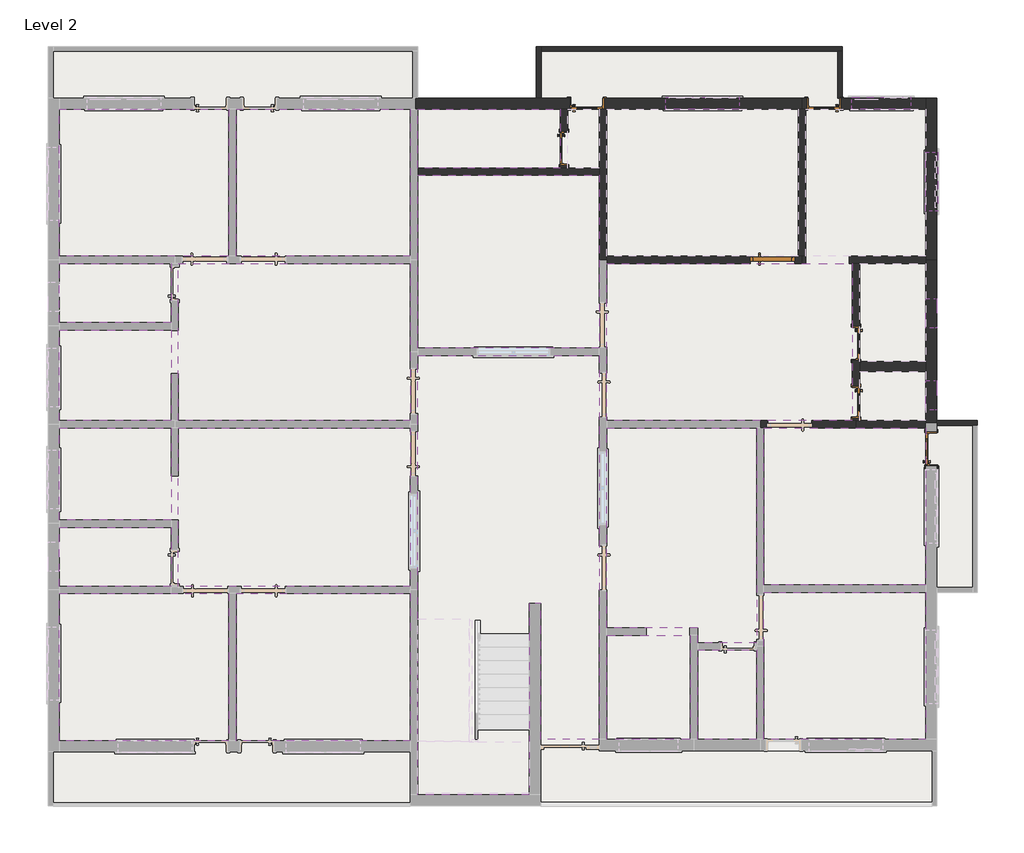
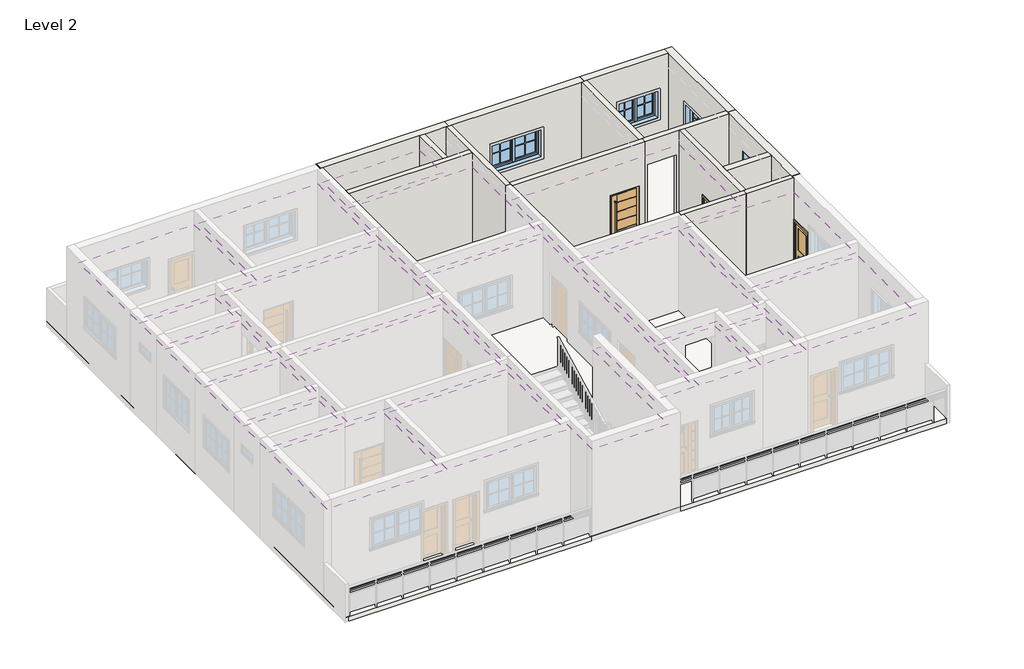
# One storey, part 3 of 5: 19 coverings, 19 walls, 7 doors, 5 windows, 1 slab.
"""IFC4 building model written with IfcOpenShell, lengths in millimetres."""

from ifc_helpers import new_model, si_unit, frame, origin, place, context, project, spatial, polyline, outline, extrude, faceted_brep, transform, mapped, element, save
from components import door_3_ad1505b7, m_door_interior_single_2_panel_wood_2_8c5b34de, door_57d9c04c, door_c5a180fb, door_5f4ff63b, door_e2914254, fixed_2_d9cafb20, m_window_awning_double_horizontal_4_0c6a2509, m_window_awning_double_horizontal_5_7c720334

model = new_model("IFC4")

# Units and contexts
model_context = context("Model", 3, world=origin())
ifc_project = project(units=[si_unit("LENGTHUNIT", "METRE", prefix="MILLI")], contexts=[model_context])

# Site, building, storey
site = spatial("IfcSite", under=ifc_project)
building = spatial("IfcBuilding", under=site)
storey = spatial("IfcBuildingStorey", under=building, Name="Level 2", Elevation=3200.4)

# Coverings
placement = place(None, origin())
element("IfcCovering", 1, ObjectType="2' x 4' ACT System", at=placement, inside=storey, context=model_context, shape_type="SweptSolid", body=[
    extrude(outline(polyline([(-22388.4847893, 20054.3922903), (-24776.0847893, 20054.3922903), (-24776.0847893, 23102.3922903), (-21270.8847893, 23102.3922903), (-21270.8847893, 20054.3922903), (-22388.4847893, 20054.3922903)])), frame((0.0, 0.0, 5943.6), z_axis=(0.0, 0.0, 1.0), x_axis=(1.0, 0.0, 0.0)), (0.0, 0.0, 1.0), 57.15),
])
element("IfcCovering", 2, ObjectType="2' x 4' ACT System", at=placement, inside=storey, context=model_context, shape_type="SweptSolid", body=[
    extrude(outline(polyline([(-21118.4847893, 23102.3922903), (-17511.6847893, 23102.3922903), (-17511.6847893, 20054.3922903), (-21118.4847893, 20054.3922903), (-21118.4847893, 23102.3922903)])), frame((0.0, 0.0, 5943.6), z_axis=(0.0, 0.0, 1.0), x_axis=(1.0, 0.0, 0.0)), (0.0, 0.0, 1.0), 57.15),
])
element("IfcCovering", 3, ObjectType="2' x 4' ACT System", at=placement, inside=storey, context=model_context, shape_type="SweptSolid", body=[
    extrude(outline(polyline([(-14412.8847893, 21883.1922903), (-17359.2847893, 21883.1922903), (-17359.2847893, 23102.3922903), (-14412.8847893, 23102.3922903), (-14412.8847893, 21883.1922903)])), frame((0.0, 0.0, 5943.6), z_axis=(0.0, 0.0, 1.0), x_axis=(1.0, 0.0, 0.0)), (0.0, 0.0, 1.0), 57.15),
])
element("IfcCovering", 4, ObjectType="2' x 4' ACT System", at=placement, inside=storey, context=model_context, shape_type="SweptSolid", body=[
    extrude(outline(polyline([(-17359.2847893, 18149.3922903), (-17359.2847893, 19978.1922903), (-17359.2847893, 21730.7922903), (-13600.0847893, 21730.7922903), (-13600.0847893, 19978.1922903), (-13600.0847893, 18149.3922903), (-17359.2847893, 18149.3922903)])), frame((0.0, 0.0, 5943.6), z_axis=(0.0, 0.0, 1.0), x_axis=(1.0, 0.0, 0.0)), (0.0, 0.0, 1.0), 57.15),
])
element("IfcCovering", 5, ObjectType="2' x 4' ACT System", at=placement, inside=storey, context=model_context, shape_type="SweptSolid", body=[
    extrude(outline(polyline([(-13447.6847893, 16650.7922903), (-13447.6847893, 19901.9922903), (-9409.0847893, 19901.9922903), (-8367.6847893, 19901.9922903), (-8367.6847893, 16650.7922903), (-10272.6847893, 16650.7922903), (-13447.6847893, 16650.7922903)])), frame((0.0, 0.0, 5943.6), z_axis=(0.0, 0.0, 1.0), x_axis=(1.0, 0.0, 0.0)), (0.0, 0.0, 1.0), 57.15),
])
element("IfcCovering", 6, ObjectType="2' x 4' ACT System", at=placement, inside=storey, context=model_context, shape_type="SweptSolid", body=[
    extrude(outline(polyline([(-6843.6847893, 16498.3922903), (-6843.6847893, 13247.1922903), (-10196.4847893, 13247.1922903), (-10196.4847893, 16498.3922903), (-8291.4847893, 16498.3922903), (-6843.6847893, 16498.3922903)])), frame((0.0, 0.0, 5943.6), z_axis=(0.0, 0.0, 1.0), x_axis=(1.0, 0.0, 0.0)), (0.0, 0.0, 1.0), 57.15),
])
element("IfcCovering", 7, ObjectType="2' x 4' ACT System", at=placement, inside=storey, context=model_context, shape_type="SweptSolid", body=[
    extrude(outline(polyline([(-6843.6847893, 13094.7922903), (-6843.6847893, 10046.7922903), (-10196.4847893, 10046.7922903), (-10196.4847893, 11977.1922903), (-10196.4847893, 13094.7922903), (-6843.6847893, 13094.7922903)])), frame((0.0, 0.0, 5943.6), z_axis=(0.0, 0.0, 1.0), x_axis=(1.0, 0.0, 0.0)), (0.0, 0.0, 1.0), 57.15),
])
element("IfcCovering", 8, ObjectType="2' x 4' ACT System", at=placement, inside=storey, context=model_context, shape_type="SweptSolid", body=[
    extrude(outline(polyline([(-11568.0847893, 10046.7922903), (-11568.0847893, 11900.9922903), (-10348.8847893, 11900.9922903), (-10348.8847893, 10046.7922903), (-11568.0847893, 10046.7922903)])), frame((0.0, 0.0, 5943.6), z_axis=(0.0, 0.0, 1.0), x_axis=(1.0, 0.0, 0.0)), (0.0, 0.0, 1.0), 57.15),
])
element("IfcCovering", 9, ObjectType="2' x 4' ACT System", at=placement, inside=storey, context=model_context, shape_type="SweptSolid", body=[
    extrude(outline(polyline([(-13447.6847893, 10046.7922903), (-13447.6847893, 12205.7922903), (-11720.4847893, 12205.7922903), (-11720.4847893, 10046.7922903), (-13447.6847893, 10046.7922903)])), frame((0.0, 0.0, 5943.6), z_axis=(0.0, 0.0, 1.0), x_axis=(1.0, 0.0, 0.0)), (0.0, 0.0, 1.0), 57.15),
])
element("IfcCovering", 10, ObjectType="2' x 4' ACT System", at=placement, inside=storey, context=model_context, shape_type="SweptSolid", body=[
    extrude(outline(polyline([(-13447.6847893, 12358.1922903), (-13447.6847893, 16498.3922903), (-10348.8847893, 16498.3922903), (-10348.8847893, 12053.3922903), (-11568.0847893, 12053.3922903), (-11568.0847893, 12358.1922903), (-13447.6847893, 12358.1922903)])), frame((0.0, 0.0, 5943.6), z_axis=(0.0, 0.0, 1.0), x_axis=(1.0, 0.0, 0.0)), (0.0, 0.0, 1.0), 57.15),
])
element("IfcCovering", 11, ObjectType="2' x 4' ACT System", at=placement, inside=storey, context=model_context, shape_type="SweptSolid", body=[
    extrude(outline(polyline([(-15047.8847893, 12866.1922903), (-15047.8847893, 8903.7922903), (-17359.2847893, 8903.7922903), (-17359.2847893, 13145.5922903), (-17359.2847893, 16574.5922903), (-17359.2847893, 17996.9922903), (-13600.0847893, 17996.9922903), (-13600.0847893, 10046.7922903), (-14819.2847893, 10046.7922903), (-14819.2847893, 12866.1922903), (-15047.8847893, 12866.1922903)])), frame((0.0, 0.0, 5943.6), z_axis=(0.0, 0.0, 1.0), x_axis=(1.0, 0.0, 0.0)), (0.0, 0.0, 1.0), 57.15),
])
element("IfcCovering", 12, ObjectType="2' x 4' ACT System", at=placement, inside=storey, context=model_context, shape_type="SweptSolid", body=[
    extrude(outline(polyline([(-17511.6847893, 13221.7922903), (-22312.2847893, 13221.7922903), (-22312.2847893, 16498.3922903), (-17511.6847893, 16498.3922903), (-17511.6847893, 13221.7922903)])), frame((0.0, 0.0, 5943.6), z_axis=(0.0, 0.0, 1.0), x_axis=(1.0, 0.0, 0.0)), (0.0, 0.0, 1.0), 57.15),
])
element("IfcCovering", 13, ObjectType="2' x 4' ACT System", at=placement, inside=storey, context=model_context, shape_type="SweptSolid", body=[
    extrude(outline(polyline([(-17511.6847893, 10021.3922903), (-21118.4847893, 10021.3922903), (-21118.4847893, 13069.3922903), (-17511.6847893, 13069.3922903), (-17511.6847893, 10021.3922903)])), frame((0.0, 0.0, 5943.6), z_axis=(0.0, 0.0, 1.0), x_axis=(1.0, 0.0, 0.0)), (0.0, 0.0, 1.0), 57.15),
])
element("IfcCovering", 14, ObjectType="2' x 4' ACT System", at=placement, inside=storey, context=model_context, shape_type="SweptSolid", body=[
    extrude(outline(polyline([(-21270.8847893, 13069.3922903), (-21270.8847893, 10021.3922903), (-24776.0847893, 10021.3922903), (-24776.0847893, 13069.3922903), (-22477.3847893, 13069.3922903), (-21270.8847893, 13069.3922903)])), frame((0.0, 0.0, 5943.6), z_axis=(0.0, 0.0, 1.0), x_axis=(1.0, 0.0, 0.0)), (0.0, 0.0, 1.0), 57.15),
])
element("IfcCovering", 15, ObjectType="2' x 4' ACT System", at=placement, inside=storey, context=model_context, shape_type="SweptSolid", body=[
    extrude(outline(polyline([(-22464.6847893, 13221.7922903), (-24776.0847893, 13221.7922903), (-24776.0847893, 14440.9922903), (-22464.6847893, 14440.9922903), (-22464.6847893, 13221.7922903)])), frame((0.0, 0.0, 5943.6), z_axis=(0.0, 0.0, 1.0), x_axis=(1.0, 0.0, 0.0)), (0.0, 0.0, 1.0), 57.15),
])
element("IfcCovering", 16, ObjectType="2' x 4' ACT System", at=placement, inside=storey, context=model_context, shape_type="SweptSolid", body=[
    extrude(outline(polyline([(-24776.0847893, 14593.3922903), (-24776.0847893, 16498.3922903), (-22464.6847893, 16498.3922903), (-22464.6847893, 14593.3922903), (-24776.0847893, 14593.3922903)])), frame((0.0, 0.0, 5943.6), z_axis=(0.0, 0.0, 1.0), x_axis=(1.0, 0.0, 0.0)), (0.0, 0.0, 1.0), 57.15),
])
element("IfcCovering", 17, ObjectType="2' x 4' ACT System", at=placement, inside=storey, context=model_context, shape_type="SweptSolid", body=[
    extrude(outline(polyline([(-22464.6847893, 18530.3922903), (-22464.6847893, 16650.7922903), (-24776.0847893, 16650.7922903), (-24776.0847893, 18530.3922903), (-22464.6847893, 18530.3922903)])), frame((0.0, 0.0, 5943.6), z_axis=(0.0, 0.0, 1.0), x_axis=(1.0, 0.0, 0.0)), (0.0, 0.0, 1.0), 57.15),
])
element("IfcCovering", 18, ObjectType="2' x 4' ACT System", at=placement, inside=storey, context=model_context, shape_type="SweptSolid", body=[
    extrude(outline(polyline([(-17511.6847893, 16650.7922903), (-22312.2847893, 16650.7922903), (-22312.2847893, 19901.9922903), (-17511.6847893, 19901.9922903), (-17511.6847893, 18073.1922903), (-17511.6847893, 16650.7922903)])), frame((0.0, 0.0, 5943.6), z_axis=(0.0, 0.0, 1.0), x_axis=(1.0, 0.0, 0.0)), (0.0, 0.0, 1.0), 57.15),
])
element("IfcCovering", 19, ObjectType="2' x 4' ACT System", at=placement, inside=storey, context=model_context, shape_type="SweptSolid", body=[
    extrude(outline(polyline([(-24776.0847893, 18682.7922903), (-24776.0847893, 19901.9922903), (-22464.6847893, 19901.9922903), (-22464.6847893, 18682.7922903), (-24776.0847893, 18682.7922903)])), frame((0.0, 0.0, 5943.6), z_axis=(0.0, 0.0, 1.0), x_axis=(1.0, 0.0, 0.0)), (0.0, 0.0, 1.0), 57.15),
])

# Doors
door_3_shape = door_3_ad1505b7(model_context)
element("IfcDoor", 20, ObjectType="3'", at=placement, inside=storey, context=model_context, shape_type="MappedRepresentation", body=[
    mapped(door_3_shape, transform((-10018.6847893, 19978.1922903, 3200.4), x_axis=(1.0, 0.0, 0.0), y_axis=(0.0, 1.0, 0.0), z_axis=(0.0, 0.0, 1.0))),
])
m_door_interior_single_2_panel_wood_2_shape = m_door_interior_single_2_panel_wood_2_8c5b34de(model_context)
element("IfcDoor", 21, ObjectType="M_Door-Interior-Single-2_Panel-Wood : 2'", at=placement, inside=storey, context=model_context, shape_type="MappedRepresentation", body=[
    mapped(m_door_interior_single_2_panel_wood_2_shape, transform((-8288.3097893, 17031.7922903, 3200.4), x_axis=(0.0, -1.0, 0.0), y_axis=(1.0, 0.0, 0.0), z_axis=(0.0, 0.0, 1.0))),
])
door_shape = door_57d9c04c(model_context)
element("IfcDoor", 22, ObjectType="M_Door-Interior-Single-2_Panel-Wood : 2'2\"", at=placement, inside=storey, context=model_context, shape_type="MappedRepresentation", body=[
    mapped(door_shape, transform((-8288.3097893, 18250.9922903, 3200.4), x_axis=(0.0, -1.0, 0.0), y_axis=(1.0, 0.0, 0.0), z_axis=(0.0, 0.0, 1.0))),
])
door_2_shape = door_c5a180fb(model_context)
element("IfcDoor", 23, ObjectType="M_Door-Interior-Single-2_Panel-Wood : 2'2\"", at=placement, inside=storey, context=model_context, shape_type="MappedRepresentation", body=[
    mapped(door_2_shape, transform((-14339.8597893, 22289.5922903, 3200.4), x_axis=(0.0, -1.0, 0.0), y_axis=(1.0, 0.0, 0.0), z_axis=(0.0, 0.0, 1.0))),
])
door_4_shape = door_5f4ff63b(model_context)
element("IfcDoor", 24, ObjectType="M_Door-Interior-Single-2_Panel-Wood : 2'2\"", at=placement, inside=storey, context=model_context, shape_type="MappedRepresentation", body=[
    mapped(door_4_shape, transform((-6732.5597893, 16066.5922903, 3200.4), x_axis=(0.0, 1.0, 0.0), y_axis=(-1.0, 0.0, 0.0), z_axis=(0.0, 0.0, 1.0))),
])
element("IfcDoor", 25, ObjectType="M_Door-Interior-Single-2_Panel-Wood : 2'2\"", at=placement, inside=storey, context=model_context, shape_type="MappedRepresentation", body=[
    mapped(door_4_shape, transform((-8951.8847893, 23213.5172903, 3200.4), x_axis=(-1.0, 0.0, 0.0), y_axis=(0.0, -1.0, 0.0), z_axis=(0.0, 0.0, 1.0))),
])
door_5_shape = door_e2914254(model_context)
element("IfcDoor", 26, ObjectType="M_Door-Interior-Single-2_Panel-Wood : 2'2\"", at=placement, inside=storey, context=model_context, shape_type="MappedRepresentation", body=[
    mapped(door_5_shape, transform((-13860.4347893, 23213.5172903, 3200.4), x_axis=(1.0, 0.0, 0.0), y_axis=(0.0, 1.0, 0.0), z_axis=(0.0, 0.0, 1.0))),
])

# Slab
element("IfcSlab", 27, ObjectType="Generic - 6\"", at=placement, inside=storey, context=model_context, shape_type="SweptSolid", body=[
    extrude(outline(polyline([(-25004.6847893, 23330.9922903), (-25004.6847893, 24397.7922903), (-21931.2847893, 24397.7922903), (-17359.2847893, 24397.7922903), (-17359.2847893, 23330.9922903), (-14902.8704844, 23330.9922903), (-14902.8704844, 24397.7922903), (-8570.8847893, 24397.7922903), (-8570.8847893, 23330.9922903), (-6615.0847893, 23330.9922903), (-6615.0847893, 19978.1922903), (-6615.0847893, 16650.7922903), (-5776.8847893, 16650.7922903), (-5776.8847893, 13094.7922903), (-6615.0847893, 13094.7922903), (-6615.0847893, 9818.1922903), (-6615.0847893, 8675.1922903), (-14819.2847893, 8675.1922903), (-17511.6847893, 8675.1922903), (-25004.6847893, 8675.1922903), (-25004.6847893, 9792.7922903), (-25004.6847893, 14517.1922903), (-25004.6847893, 18606.5922903), (-25004.6847893, 23330.9922903)])), frame((0.0, 0.0, 3200.4), z_axis=(0.0, 0.0, 1.0), x_axis=(1.0, 0.0, 0.0)), (0.0, 0.0, 1.0), 152.4),
])

# Walls
element("IfcWall", 28, ObjectType="Generic - 4\"", at=placement, inside=storey, context=model_context, shape_type="Brep", body=[
    faceted_brep([(-14801.2704844, 23330.9922903, 3200.4), (-14801.2704844, 24296.1922903, 3200.4), (-14801.2704844, 24397.7922903, 3200.4), (-14801.2704844, 24397.7922903, 4419.6), (-14801.2704844, 24296.1922903, 4419.6), (-14801.2704844, 23330.9922903, 4419.6), (-14902.8704844, 23330.9922903, 3200.4), (-14902.8704844, 23330.9922903, 4419.6), (-14902.8704844, 24397.7922903, 4419.6), (-14902.8704844, 24397.7922903, 3200.4)], [[[0, 1, 2, 3, 4, 5]], [[6, 7, 8, 9]], [[2, 1, 0, 6, 9]], [[5, 4, 3, 8, 7]], [[0, 5, 7, 6]], [[3, 2, 9, 8]]]),
])
element("IfcWall", 29, ObjectType="Generic - 4\"", at=placement, inside=storey, context=model_context, shape_type="Brep", body=[
    faceted_brep([(-14801.2704844, 24296.1922903, 3200.4), (-8672.4847893, 24296.1922903, 3200.4), (-8570.8847893, 24296.1922903, 3200.4), (-8570.8847893, 24296.1922903, 4419.6), (-8672.4847893, 24296.1922903, 4419.6), (-14801.2704844, 24296.1922903, 4419.6), (-14801.2704844, 24397.7922903, 3200.4), (-14801.2704844, 24397.7922903, 4419.6), (-8570.8847893, 24397.7922903, 4419.6), (-8570.8847893, 24397.7922903, 3200.4)], [[[0, 1, 2, 3, 4, 5]], [[6, 7, 8, 9]], [[2, 1, 0, 6, 9]], [[5, 4, 3, 8, 7]], [[0, 5, 7, 6]], [[3, 2, 9, 8]]]),
])
element("IfcWall", 30, ObjectType="Generic - 4\"", at=placement, inside=storey, context=model_context, shape_type="Brep", body=[
    faceted_brep([(-8672.4847893, 24296.1922903, 3200.4), (-8672.4847893, 23330.9922903, 3200.4), (-8672.4847893, 23330.9922903, 4419.6), (-8672.4847893, 24296.1922903, 4419.6), (-8570.8847893, 24296.1922903, 3200.4), (-8570.8847893, 24296.1922903, 4419.6), (-8570.8847893, 23330.9922903, 4419.6), (-8570.8847893, 23330.9922903, 3200.4), (-8596.6847893, 23330.9922903, 3200.4)], [[[0, 1, 2, 3]], [[4, 5, 6, 7]], [[1, 0, 4, 7, 8]], [[3, 2, 6, 5]], [[0, 3, 5, 4]], [[2, 1, 8, 7, 6]]]),
])
element("IfcWall", 31, ObjectType="Generic - 4\"", at=placement, inside=storey, context=model_context, shape_type="Brep", body=[
    faceted_brep([(-6615.0847893, 16549.1922903, 3200.4), (-5878.4847893, 16549.1922903, 3200.4), (-5776.8847893, 16549.1922903, 3200.4), (-5776.8847893, 16549.1922903, 4419.6), (-5878.4847893, 16549.1922903, 4419.6), (-6615.0847893, 16549.1922903, 4419.6), (-6615.0847893, 16650.7922903, 3200.4), (-6615.0847893, 16650.7922903, 4419.6), (-5776.8847893, 16650.7922903, 4419.6), (-5776.8847893, 16650.7922903, 3200.4), (-6615.0847893, 16574.5922903, 3200.4), (-6615.0847893, 16599.9922903, 3200.4)], [[[0, 1, 2, 3, 4, 5]], [[6, 7, 8, 9]], [[2, 1, 0, 10, 11, 6, 9]], [[5, 4, 3, 8, 7]], [[0, 5, 7, 6, 11, 10]], [[3, 2, 9, 8]]]),
])
element("IfcWall", 32, ObjectType="Generic - 6\"", at=placement, inside=storey, context=model_context, shape_type="Brep", body=[
    faceted_brep([(-13600.0847893, 19978.1922903, 3200.4), (-13600.0847893, 19978.1922903, 6400.8), (-13600.0847893, 21730.7922903, 6400.8), (-13600.0847893, 21883.1922903, 6400.8), (-13600.0847893, 23102.3922903, 6400.8), (-13600.0847893, 23102.3922903, 3200.4), (-13600.0847893, 21883.1922903, 3200.4), (-13600.0847893, 21883.1922903, 3347.5515697), (-13600.0847893, 21730.7922903, 3347.5515697), (-13600.0847893, 21730.7922903, 3200.4), (-13447.6847893, 19978.1922903, 3200.4), (-13447.6847893, 20054.3922903, 3200.4), (-13447.6847893, 23102.3922903, 3200.4), (-13447.6847893, 23102.3922903, 6400.8), (-13447.6847893, 20054.3922903, 6400.8), (-13447.6847893, 19978.1922903, 6400.8), (-13536.9847893, 21730.7922903, 3200.4), (-13536.9847893, 21883.1922903, 3200.4), (-13523.8847893, 23102.3922903, 3200.4), (-13505.2347893, 23102.3922903, 3200.4), (-13523.8847893, 23102.3922903, 6400.8), (-13536.9847893, 21730.7922903, 3347.5515697), (-13536.9847893, 21883.1922903, 3347.5515697)], [[[0, 1, 2, 3, 4, 5, 6, 7, 8, 9]], [[10, 11, 12, 13, 14, 15]], [[12, 11, 10, 0, 9, 16, 17, 6, 5, 18, 19]], [[1, 0, 10, 15]], [[4, 3, 2, 1, 15, 14, 13, 20]], [[5, 4, 20, 13, 12, 19, 18]], [[8, 21, 16, 9]], [[17, 22, 7, 6]], [[22, 21, 8, 7]], [[21, 22, 17, 16]]]),
])
element("IfcWall", 33, ObjectType="Generic - 6\"", at=placement, inside=storey, context=model_context, shape_type="Brep", body=[
    faceted_brep([(-13600.0847893, 21730.7922903, 6400.8), (-17359.2847893, 21730.7922903, 6400.8), (-17359.2847893, 21730.7922903, 3200.4), (-14247.3847893, 21730.7922903, 3200.4), (-14247.3847893, 21730.7922903, 3347.5515697), (-13600.0847893, 21730.7922903, 3347.5515697), (-17359.2847893, 21883.1922903, 6400.8), (-14412.8847893, 21883.1922903, 6400.8), (-14260.4847893, 21883.1922903, 6400.8), (-13600.0847893, 21883.1922903, 6400.8), (-13600.0847893, 21883.1922903, 3347.5515697), (-14247.3847893, 21883.1922903, 3347.5515697), (-14247.3847893, 21883.1922903, 3200.4), (-14260.4847893, 21883.1922903, 3200.4), (-14412.8847893, 21883.1922903, 3200.4), (-17359.2847893, 21883.1922903, 3200.4)], [[[0, 1, 2, 3, 4, 5]], [[6, 7, 8, 9, 10, 11, 12, 13, 14, 15]], [[2, 15, 14, 13, 12, 3]], [[1, 0, 9, 8, 7, 6]], [[2, 1, 6, 15]], [[9, 0, 5, 10]], [[4, 11, 10, 5]], [[11, 4, 3, 12]]]),
])
element("IfcWall", 34, ObjectType="Generic - 6\"", at=placement, inside=storey, context=model_context, shape_type="Brep", body=[
    faceted_brep([(-9409.0847893, 19901.9922903, 3200.4), (-9409.0847893, 19901.9922903, 6400.8), (-13447.6847893, 19901.9922903, 6400.8), (-13447.6847893, 19901.9922903, 3200.4), (-10475.8847893, 19901.9922903, 3200.4), (-10475.8847893, 19901.9922903, 5029.2), (-9561.4847893, 19901.9922903, 5029.2), (-9561.4847893, 19901.9922903, 3200.4), (-9409.0847893, 20054.3922903, 6400.8), (-9409.0847893, 20054.3922903, 3200.4), (-9485.2847893, 20054.3922903, 3200.4), (-9561.4847893, 20054.3922903, 3200.4), (-9561.4847893, 20054.3922903, 5029.2), (-10475.8847893, 20054.3922903, 5029.2), (-10475.8847893, 20054.3922903, 3200.4), (-13447.6847893, 20054.3922903, 3200.4), (-13447.6847893, 20054.3922903, 6400.8), (-9485.2847893, 20054.3922903, 6400.8), (-13447.6847893, 19978.1922903, 3200.4), (-10475.8847893, 20034.3922903, 3200.4), (-10490.8847893, 20034.3922903, 3200.4), (-10490.8847893, 19957.3922903, 3200.4), (-10475.8847893, 19957.3922903, 3200.4), (-9561.4847893, 19957.3922903, 3200.4), (-9546.4847893, 19957.3922903, 3200.4), (-9546.4847893, 20034.3922903, 3200.4), (-9561.4847893, 20034.3922903, 3200.4), (-13447.6847893, 19978.1922903, 6400.8), (-9561.4847893, 20034.3922903, 5029.2), (-10475.8847893, 20034.3922903, 5029.2), (-10475.8847893, 19957.3922903, 5029.2), (-9561.4847893, 19957.3922903, 5029.2), (-10490.8847893, 20034.3922903, 5044.2), (-9546.4847893, 20034.3922903, 5044.2), (-9546.4847893, 19957.3922903, 5044.2), (-10490.8847893, 19957.3922903, 5044.2)], [[[0, 1, 2, 3, 4, 5, 6, 7]], [[8, 9, 10, 11, 12, 13, 14, 15, 16, 17]], [[3, 18, 15, 14, 19, 20, 21, 22, 4]], [[9, 0, 7, 23, 24, 25, 26, 11, 10]], [[1, 0, 9, 8]], [[2, 1, 8, 17, 16, 27]], [[3, 2, 27, 16, 15, 18]], [[12, 28, 29, 13]], [[5, 30, 31, 6]], [[28, 12, 11, 26]], [[6, 31, 23, 7]], [[13, 29, 19, 14]], [[30, 5, 4, 22]], [[32, 33, 34, 35]], [[34, 33, 25, 24]], [[31, 30, 22, 21, 35, 34, 24, 23]], [[32, 35, 21, 20]], [[29, 28, 26, 25, 33, 32, 20, 19]]]),
])
element("IfcWall", 35, ObjectType="Generic - 6\"", at=placement, inside=storey, context=model_context, shape_type="Brep", body=[
    faceted_brep([(-9485.2847893, 23102.3922903, 3200.4), (-9485.2847893, 20054.3922903, 3200.4), (-9485.2847893, 20054.3922903, 6400.8), (-9485.2847893, 23102.3922903, 6400.8), (-9332.8847893, 23102.3922903, 3200.4), (-9332.8847893, 23102.3922903, 6400.8), (-9332.8847893, 20054.3922903, 6400.8), (-9332.8847893, 20054.3922903, 5638.8), (-9332.8847893, 20054.3922903, 3200.4), (-9409.0847893, 23102.3922903, 3200.4), (-9409.0847893, 20054.3922903, 3200.4), (-9409.0847893, 20054.3922903, 6400.8), (-9409.0847893, 23102.3922903, 6400.8)], [[[0, 1, 2, 3]], [[4, 5, 6, 7, 8]], [[1, 0, 9, 4, 8, 10]], [[3, 2, 11, 6, 5, 12]], [[0, 3, 12, 5, 4, 9]], [[2, 1, 10, 8, 7, 6, 11]]]),
])
element("IfcWall", 36, ObjectType="Generic - 6\"", at=placement, inside=storey, context=model_context, shape_type="Brep", body=[
    faceted_brep([(-8367.6847893, 16650.7922903, 6400.8), (-8367.6847893, 19901.9922903, 6400.8), (-8367.6847893, 19901.9922903, 3200.4), (-8367.6847893, 18606.1922903, 3200.4), (-8367.6847893, 18606.1922903, 5054.2), (-8367.6847893, 17895.7922903, 5054.2), (-8367.6847893, 17895.7922903, 3200.4), (-8367.6847893, 17361.5922903, 3200.4), (-8367.6847893, 17361.5922903, 5054.2), (-8367.6847893, 16701.9922903, 5054.2), (-8367.6847893, 16701.9922903, 3200.4), (-8367.6847893, 16650.7922903, 3200.4), (-8215.2847893, 19901.9922903, 6400.8), (-8215.2847893, 17869.9922903, 6400.8), (-8215.2847893, 17666.7922903, 6400.8), (-8215.2847893, 16650.7922903, 6400.8), (-8215.2847893, 16650.7922903, 3200.4), (-8215.2847893, 16701.9922903, 3200.4), (-8215.2847893, 16701.9922903, 5054.2), (-8215.2847893, 17361.5922903, 5054.2), (-8215.2847893, 17361.5922903, 3200.4), (-8215.2847893, 17666.7922903, 3200.4), (-8215.2847893, 17869.9922903, 3200.4), (-8215.2847893, 17895.7922903, 3200.4), (-8215.2847893, 17895.7922903, 5054.2), (-8215.2847893, 18606.1922903, 5054.2), (-8215.2847893, 18606.1922903, 3200.4), (-8215.2847893, 19901.9922903, 3200.4), (-8291.4847893, 16650.7922903, 3200.4), (-8291.4847893, 16650.7922903, 6400.8)], [[[0, 1, 2, 3, 4, 5, 6, 7, 8, 9, 10, 11]], [[12, 13, 14, 15, 16, 17, 18, 19, 20, 21, 22, 23, 24, 25, 26, 27]], [[2, 27, 26, 3]], [[16, 28, 11, 10, 17]], [[20, 7, 6, 23, 22, 21]], [[1, 0, 29, 15, 14, 13, 12]], [[2, 1, 12, 27]], [[0, 11, 28, 16, 15, 29]], [[9, 18, 17, 10]], [[18, 9, 8, 19]], [[19, 8, 7, 20]], [[5, 24, 23, 6]], [[24, 5, 4, 25]], [[25, 4, 3, 26]]]),
])
element("IfcWall", 37, ObjectType="Generic - 6\"", at=placement, inside=storey, context=model_context, shape_type="Brep", body=[
    faceted_brep([(-8291.4847893, 16498.3922903, 3200.4), (-8291.4847893, 16498.3922903, 6400.8), (-10196.4847893, 16498.3922903, 6400.8), (-10272.6847893, 16498.3922903, 6400.8), (-10272.6847893, 16498.3922903, 3200.4), (-10196.4847893, 16498.3922903, 3200.4), (-10120.2847893, 16498.3922903, 3200.4), (-10120.2847893, 16498.3922903, 5029.2), (-9205.8847893, 16498.3922903, 5029.2), (-9205.8847893, 16498.3922903, 3200.4), (-8291.4847893, 16650.7922903, 6400.8), (-8291.4847893, 16650.7922903, 3200.4), (-8367.6847893, 16650.7922903, 3200.4), (-9205.8847893, 16650.7922903, 3200.4), (-9205.8847893, 16650.7922903, 5029.2), (-10120.2847893, 16650.7922903, 5029.2), (-10120.2847893, 16650.7922903, 3200.4), (-10272.6847893, 16650.7922903, 3200.4), (-10272.6847893, 16650.7922903, 6400.8), (-8367.6847893, 16650.7922903, 6400.8), (-10120.2847893, 16595.3922903, 3200.4), (-10135.2847893, 16595.3922903, 3200.4), (-10135.2847893, 16518.3922903, 3200.4), (-10120.2847893, 16518.3922903, 3200.4), (-9205.8847893, 16518.3922903, 3200.4), (-9190.8847893, 16518.3922903, 3200.4), (-9190.8847893, 16595.3922903, 3200.4), (-9205.8847893, 16595.3922903, 3200.4), (-9205.8847893, 16595.3922903, 5029.2), (-10120.2847893, 16595.3922903, 5029.2), (-10120.2847893, 16518.3922903, 5029.2), (-9205.8847893, 16518.3922903, 5029.2), (-9190.8847893, 16518.3922903, 5044.2), (-10135.2847893, 16518.3922903, 5044.2), (-10135.2847893, 16595.3922903, 5044.2), (-9190.8847893, 16595.3922903, 5044.2)], [[[0, 1, 2, 3, 4, 5, 6, 7, 8, 9]], [[10, 11, 12, 13, 14, 15, 16, 17, 18, 19]], [[4, 17, 16, 20, 21, 22, 23, 6, 5]], [[11, 0, 9, 24, 25, 26, 27, 13, 12]], [[1, 0, 11, 10]], [[3, 2, 1, 10, 19, 18]], [[4, 3, 18, 17]], [[14, 28, 29, 15]], [[7, 30, 31, 8]], [[15, 29, 20, 16]], [[30, 7, 6, 23]], [[28, 14, 13, 27]], [[8, 31, 24, 9]], [[32, 33, 34, 35]], [[34, 33, 22, 21]], [[29, 28, 27, 26, 35, 34, 21, 20]], [[32, 35, 26, 25]], [[31, 30, 23, 22, 33, 32, 25, 24]]]),
])
element("IfcWall", 38, ObjectType="Generic - 6\"", at=placement, inside=storey, context=model_context, shape_type="Brep", body=[
    faceted_brep([(-6843.6847893, 19901.9922903, 3200.4), (-6843.6847893, 19901.9922903, 6400.8), (-8215.2847893, 19901.9922903, 6400.8), (-8367.6847893, 19901.9922903, 6400.8), (-9409.0847893, 19901.9922903, 6400.8), (-9409.0847893, 19901.9922903, 3200.4), (-9332.8847893, 19901.9922903, 3200.4), (-9332.8847893, 19901.9922903, 5638.8), (-8430.9142678, 19901.9922903, 5638.8), (-8430.9142678, 19901.9922903, 3200.4), (-8367.6847893, 19901.9922903, 3200.4), (-8215.2847893, 19901.9922903, 3200.4), (-6843.6847893, 20054.3922903, 6400.8), (-6843.6847893, 20054.3922903, 3200.4), (-8430.9142678, 20054.3922903, 3200.4), (-8430.9142678, 20054.3922903, 5638.8), (-9332.8847893, 20054.3922903, 5638.8), (-9332.8847893, 20054.3922903, 3200.4), (-9409.0847893, 20054.3922903, 3200.4), (-9409.0847893, 20054.3922903, 6400.8), (-9332.8847893, 20054.3922903, 6400.8), (-6843.6847893, 19978.1922903, 3200.4), (-6843.6847893, 19978.1922903, 6400.8)], [[[0, 1, 2, 3, 4, 5, 6, 7, 8, 9, 10, 11]], [[12, 13, 14, 15, 16, 17, 18, 19, 20]], [[13, 21, 0, 11, 10, 9, 14]], [[5, 18, 17, 6]], [[4, 3, 2, 1, 22, 12, 20, 19]], [[5, 4, 19, 18]], [[1, 0, 21, 13, 12, 22]], [[7, 16, 15, 8]], [[16, 7, 6, 17]], [[8, 15, 14, 9]]]),
])
element("IfcWall", 39, ObjectType="Generic - 6\"", at=placement, inside=storey, context=model_context, shape_type="Brep", body=[
    faceted_brep([(-8291.4847893, 16498.3922903, 3200.4), (-6843.6847893, 16498.3922903, 3200.4), (-6843.6847893, 16498.3922903, 6400.8), (-8291.4847893, 16498.3922903, 6400.8), (-8291.4847893, 16650.7922903, 3200.4), (-8291.4847893, 16650.7922903, 6400.8), (-8215.2847893, 16650.7922903, 6400.8), (-6843.6847893, 16650.7922903, 6400.8), (-6843.6847893, 16650.7922903, 3200.4), (-8215.2847893, 16650.7922903, 3200.4), (-6843.6847893, 16599.9922903, 3200.4), (-6843.6847893, 16574.5922903, 3200.4), (-6843.6847893, 16574.5922903, 6400.8), (-6843.6847893, 16599.9922903, 6400.8)], [[[0, 1, 2, 3]], [[4, 5, 6, 7, 8, 9]], [[1, 0, 4, 9, 8, 10, 11]], [[3, 2, 12, 13, 7, 6, 5]], [[0, 3, 5, 4]], [[1, 11, 10, 8, 7, 13, 12, 2]]]),
])
element("IfcWall", 40, ObjectType="Generic - 6\"", at=placement, inside=storey, context=model_context, shape_type="SweptSolid", body=[
    extrude(outline(polyline([(21883.1922903, 6400.8), (23102.3922903, 6400.8), (23102.3922903, 3200.4), (22644.7922903, 3200.4), (22644.7922903, 5054.2), (21934.3922903, 5054.2), (21934.3922903, 3200.4), (21883.1922903, 3200.4), (21883.1922903, 6400.8)])), frame((-14412.8847893, 0.0, 0.0), z_axis=(1.0, 0.0, 0.0), x_axis=(0.0, 1.0, 0.0)), (0.0, 0.0, 1.0), 152.4),
])
element("IfcWall", 41, ObjectType="Generic - 8\"", at=placement, inside=storey, context=model_context, shape_type="SweptSolid", body=[
    extrude(outline(polyline([(-6843.6847893, 17666.7922903), (-8215.2847893, 17666.7922903), (-8215.2847893, 17869.9922903), (-6843.6847893, 17869.9922903), (-6843.6847893, 17666.7922903)])), frame((0.0, 0.0, 3200.4), z_axis=(0.0, 0.0, 1.0), x_axis=(1.0, 0.0, 0.0)), (0.0, 0.0, 1.0), 3200.4),
])
element("IfcWall", 42, ObjectType="Generic - 9\"", at=placement, inside=storey, context=model_context, shape_type="Brep", body=[
    faceted_brep([(-9409.0847893, 23330.9922903, 3200.4), (-9409.0847893, 23330.9922903, 6400.8), (-6843.6847893, 23330.9922903, 6400.8), (-6843.6847893, 23330.9922903, 3200.4), (-8570.8847893, 23330.9922903, 3200.4), (-8596.6847893, 23330.9922903, 3200.4), (-8596.6847893, 23330.9922903, 5054.2), (-9307.0847893, 23330.9922903, 5054.2), (-9307.0847893, 23330.9922903, 3200.4), (-7154.8347893, 23330.9922903, 5334.0), (-8374.0347893, 23330.9922903, 5334.0), (-8374.0347893, 23330.9922903, 4419.6), (-7154.8347893, 23330.9922903, 4419.6), (-9409.0847893, 23102.3922903, 6400.8), (-9409.0847893, 23102.3922903, 3200.4), (-9332.8847893, 23102.3922903, 3200.4), (-9307.0847893, 23102.3922903, 3200.4), (-9307.0847893, 23102.3922903, 5054.2), (-8596.6847893, 23102.3922903, 5054.2), (-8596.6847893, 23102.3922903, 3200.4), (-6843.6847893, 23102.3922903, 3200.4), (-6843.6847893, 23102.3922903, 6400.8), (-9332.8847893, 23102.3922903, 6400.8), (-7154.8347893, 23102.3922903, 5334.0), (-7154.8347893, 23102.3922903, 4419.6), (-8374.0347893, 23102.3922903, 4419.6), (-8374.0347893, 23102.3922903, 5334.0)], [[[0, 1, 2, 3, 4, 5, 6, 7, 8], [9, 10, 11, 12]], [[13, 14, 15, 16, 17, 18, 19, 20, 21, 22], [23, 24, 25, 26]], [[3, 20, 19, 5, 4]], [[14, 0, 8, 16, 15]], [[1, 0, 14, 13]], [[2, 1, 13, 22, 21]], [[3, 2, 21, 20]], [[24, 23, 9, 12]], [[25, 24, 12, 11]], [[26, 25, 11, 10]], [[23, 26, 10, 9]], [[7, 17, 16, 8]], [[17, 7, 6, 18]], [[18, 6, 5, 19]]]),
])
element("IfcWall", 43, ObjectType="Generic - 9\"", at=placement, inside=storey, context=model_context, shape_type="Brep", body=[
    faceted_brep([(-17435.4847893, 23330.9922903, 6400.8), (-13523.8847893, 23330.9922903, 6400.8), (-13523.8847893, 23330.9922903, 5054.2), (-14215.6347893, 23330.9922903, 5054.2), (-14215.6347893, 23330.9922903, 3200.4), (-14801.2704844, 23330.9922903, 3200.4), (-14902.8704844, 23330.9922903, 3200.4), (-17359.2847893, 23330.9922903, 3200.4), (-17435.4847893, 23330.9922903, 3200.4), (-13523.8847893, 23102.3922903, 6400.8), (-13600.0847893, 23102.3922903, 6400.8), (-14260.4847893, 23102.3922903, 6400.8), (-14412.8847893, 23102.3922903, 6400.8), (-17359.2847893, 23102.3922903, 6400.8), (-17435.4847893, 23102.3922903, 6400.8), (-17435.4847893, 23102.3922903, 3200.4), (-17359.2847893, 23102.3922903, 3200.4), (-14412.8847893, 23102.3922903, 3200.4), (-14260.4847893, 23102.3922903, 3200.4), (-14215.6347893, 23102.3922903, 3200.4), (-14215.6347893, 23102.3922903, 5054.2), (-13523.8847893, 23102.3922903, 5054.2)], [[[0, 1, 2, 3, 4, 5, 6, 7, 8]], [[9, 10, 11, 12, 13, 14, 15, 16, 17, 18, 19, 20, 21]], [[15, 8, 7, 6, 5, 4, 19, 18, 17, 16]], [[1, 0, 14, 13, 12, 11, 10, 9]], [[1, 9, 21, 2]], [[20, 3, 2, 21]], [[3, 20, 19, 4]], [[8, 15, 14, 0]]]),
])
element("IfcWall", 44, ObjectType="Generic - 9\"", at=placement, inside=storey, context=model_context, shape_type="Brep", body=[
    faceted_brep([(-13523.8847893, 23330.9922903, 6400.8), (-9409.0847893, 23330.9922903, 6400.8), (-9409.0847893, 23330.9922903, 3200.4), (-13505.2347893, 23330.9922903, 3200.4), (-13505.2347893, 23330.9922903, 5054.2), (-13523.8847893, 23330.9922903, 5054.2), (-10704.4847893, 23330.9922903, 5333.9570313), (-12228.4847893, 23330.9922903, 5333.9570313), (-12228.4847893, 23330.9922903, 4419.5570313), (-10704.4847893, 23330.9922903, 4419.5570313), (-9409.0847893, 23102.3922903, 6400.8), (-9485.2847893, 23102.3922903, 6400.8), (-13447.6847893, 23102.3922903, 6400.8), (-13523.8847893, 23102.3922903, 6400.8), (-13523.8847893, 23102.3922903, 5054.2), (-13505.2347893, 23102.3922903, 5054.2), (-13505.2347893, 23102.3922903, 3200.4), (-13447.6847893, 23102.3922903, 3200.4), (-9485.2847893, 23102.3922903, 3200.4), (-9409.0847893, 23102.3922903, 3200.4), (-12228.4847893, 23102.3922903, 5333.9570313), (-10704.4847893, 23102.3922903, 5333.9570313), (-10704.4847893, 23102.3922903, 4419.5570313), (-12228.4847893, 23102.3922903, 4419.5570313)], [[[0, 1, 2, 3, 4, 5], [6, 7, 8, 9]], [[10, 11, 12, 13, 14, 15, 16, 17, 18, 19], [20, 21, 22, 23]], [[2, 19, 18, 17, 16, 3]], [[13, 0, 5, 14]], [[1, 0, 13, 12, 11, 10]], [[2, 1, 10, 19]], [[21, 20, 7, 6]], [[20, 23, 8, 7]], [[23, 22, 9, 8]], [[22, 21, 6, 9]], [[15, 4, 3, 16]], [[4, 15, 14, 5]]]),
])
element("IfcWall", 45, ObjectType="Generic - 9\"", at=placement, inside=storey, context=model_context, shape_type="Brep", body=[
    faceted_brep([(-6615.0847893, 19978.1922903, 3200.4), (-6615.0847893, 23330.9922903, 3200.4), (-6615.0847893, 23330.9922903, 6400.8), (-6615.0847893, 19978.1922903, 6400.8), (-6615.0847893, 20987.8422903, 5334.0), (-6615.0847893, 22207.0422903, 5334.0), (-6615.0847893, 22207.0422903, 4419.6), (-6615.0847893, 20987.8422903, 4419.6), (-6843.6847893, 19978.1922903, 3200.4), (-6843.6847893, 19978.1922903, 6400.8), (-6843.6847893, 20054.3922903, 6400.8), (-6843.6847893, 23102.3922903, 6400.8), (-6843.6847893, 23330.9922903, 6400.8), (-6843.6847893, 23330.9922903, 3200.4), (-6843.6847893, 23102.3922903, 3200.4), (-6843.6847893, 20054.3922903, 3200.4), (-6843.6847893, 20987.8422903, 5334.0), (-6843.6847893, 20987.8422903, 4419.6), (-6843.6847893, 22207.0422903, 4419.6), (-6843.6847893, 22207.0422903, 5334.0)], [[[0, 1, 2, 3], [4, 5, 6, 7]], [[8, 9, 10, 11, 12, 13, 14, 15], [16, 17, 18, 19]], [[1, 0, 8, 15, 14, 13]], [[3, 2, 12, 11, 10, 9]], [[0, 3, 9, 8]], [[2, 1, 13, 12]], [[16, 19, 5, 4]], [[19, 18, 6, 5]], [[18, 17, 7, 6]], [[17, 16, 4, 7]]]),
])
element("IfcWall", 46, ObjectType="Generic - 9\"", at=placement, inside=storey, context=model_context, shape_type="Brep", body=[
    faceted_brep([(-6615.0847893, 16574.5922903, 6400.8), (-6615.0847893, 16574.5922903, 3200.4), (-6615.0847893, 16650.7922903, 3200.4), (-6615.0847893, 19978.1922903, 3200.4), (-6615.0847893, 19978.1922903, 6400.8), (-6615.0847893, 16866.6922903, 5638.8), (-6615.0847893, 17476.2922903, 5638.8), (-6615.0847893, 17476.2922903, 5334.0), (-6615.0847893, 16866.6922903, 5334.0), (-6615.0847893, 18568.4922903, 5638.8), (-6615.0847893, 19178.0922903, 5638.8), (-6615.0847893, 19178.0922903, 5334.0), (-6615.0847893, 18568.4922903, 5334.0), (-6843.6847893, 16574.5922903, 3200.4), (-6843.6847893, 16574.5922903, 6400.8), (-6843.6847893, 16650.7922903, 6400.8), (-6843.6847893, 17666.7922903, 6400.8), (-6843.6847893, 17869.9922903, 6400.8), (-6843.6847893, 19901.9922903, 6400.8), (-6843.6847893, 19978.1922903, 6400.8), (-6843.6847893, 19978.1922903, 3200.4), (-6843.6847893, 19901.9922903, 3200.4), (-6843.6847893, 17869.9922903, 3200.4), (-6843.6847893, 17666.7922903, 3200.4), (-6843.6847893, 16650.7922903, 3200.4), (-6843.6847893, 16866.6922903, 5638.8), (-6843.6847893, 16866.6922903, 5334.0), (-6843.6847893, 17476.2922903, 5334.0), (-6843.6847893, 17476.2922903, 5638.8), (-6843.6847893, 18568.4922903, 5638.8), (-6843.6847893, 18568.4922903, 5334.0), (-6843.6847893, 19178.0922903, 5334.0), (-6843.6847893, 19178.0922903, 5638.8)], [[[0, 1, 2, 3, 4], [5, 6, 7, 8], [9, 10, 11, 12]], [[13, 14, 15, 16, 17, 18, 19, 20, 21, 22, 23, 24], [25, 26, 27, 28], [29, 30, 31, 32]], [[3, 2, 1, 13, 24, 23, 22, 21, 20]], [[4, 3, 20, 19]], [[0, 4, 19, 18, 17, 16, 15, 14]], [[25, 28, 6, 5]], [[28, 27, 7, 6]], [[27, 26, 8, 7]], [[26, 25, 5, 8]], [[29, 32, 10, 9]], [[32, 31, 11, 10]], [[31, 30, 12, 11]], [[30, 29, 9, 12]], [[0, 14, 13, 1]]]),
])

# Windows
fixed_2_shape = fixed_2_d9cafb20(model_context)
element("IfcWindow", 47, ObjectType="Fixed : 2'", at=placement, inside=storey, context=model_context, shape_type="MappedRepresentation", body=[
    mapped(fixed_2_shape, transform((-6729.3847893, 17133.3922903, 3200.4), x_axis=(0.0, -1.0, 0.0), y_axis=(1.0, 0.0, 0.0), z_axis=(0.0, 0.0, 1.0))),
])
element("IfcWindow", 48, ObjectType="Fixed : 2'", at=placement, inside=storey, context=model_context, shape_type="MappedRepresentation", body=[
    mapped(fixed_2_shape, transform((-6729.3847893, 18835.1922903, 3200.4), x_axis=(0.0, -1.0, 0.0), y_axis=(1.0, 0.0, 0.0), z_axis=(0.0, 0.0, 1.0))),
])
m_window_awning_double_horizontal_4_shape = m_window_awning_double_horizontal_4_0c6a2509(model_context)
element("IfcWindow", 49, ObjectType="M_Window-Awning-Double-Horizontal : 4'", at=placement, inside=storey, context=model_context, shape_type="MappedRepresentation", body=[
    mapped(m_window_awning_double_horizontal_4_shape, transform((-6729.3847893, 21597.4422903, 3519.6), x_axis=(0.0, -1.0, 0.0), y_axis=(1.0, 0.0, 0.0), z_axis=(0.0, 0.0, 1.0))),
])
element("IfcWindow", 50, ObjectType="M_Window-Awning-Double-Horizontal : 4'", at=placement, inside=storey, context=model_context, shape_type="MappedRepresentation", body=[
    mapped(m_window_awning_double_horizontal_4_shape, transform((-7764.4347893, 23216.6922903, 3519.6), x_axis=(1.0, 0.0, 0.0), y_axis=(0.0, 1.0, 0.0), z_axis=(0.0, 0.0, 1.0))),
])
m_window_awning_double_horizontal_5_shape = m_window_awning_double_horizontal_5_7c720334(model_context)
element("IfcWindow", 51, ObjectType="M_Window-Awning-Double-Horizontal : 5'", at=placement, inside=storey, context=model_context, shape_type="MappedRepresentation", body=[
    mapped(m_window_awning_double_horizontal_5_shape, transform((-11466.4847893, 23216.6922903, 3519.5570312), x_axis=(1.0, 0.0, 0.0), y_axis=(0.0, 1.0, 0.0), z_axis=(0.0, 0.0, 1.0))),
])

save(model, "model.ifc")

# Revit data of these elements
# Type "2' x 4' ACT System"
#   Assembly Code = "C3030210"
#   built-in parameter 1002203 = 1 (stored number, unit not read)
#   built-in parameter 1002202 = 1 (stored number, unit not read)
#   Layers, outside or top first: 0' - 1 5/8" "Default" (function 1); 0' - 0 5/8" "Acoustic Ceiling Tile 24 x 48" (function 5)
# Type "3'"
#   Type Mark = "9"
#   Water resistance = "up to Class E900, EN 12208:2001"
#   Uniclass2015Version = "v1.21"
#   Uniclass2015Reference = "Ss_25_30_20_30"
#   Uniclass2015Description = "Frame and door leaf system"
#   URL = "www.aluprof.com"
#   Type IFC Predefined Type = "USERDEFINED"
#   Right-hand / Left-hand door [instance default] = ""
#   Resistance to wind load = "up to Class C5/B5, EN 12210:2001"
#   Insert type = "ST"
#   Hardware [instance default] = ""
#   Product page = "https://aluprof.com/en/architects/offer/window-and-door-systems/panel-doors#visualisation"
#   Operation = "SinglePanelOutwardOpening"
#   Opening type = "Outward"
#   NBSReference = "25-50-20/125"
#   NBSDescription = "Frame and door leaf system"
#   Important = "The actual acceptable construction dimensions are dependent on the selection of profiles and hardware, glazing type, construction weight and the construction’s operating conditions. These should be determined by a suitably qualified person, and using ALUPROF’s calculation software"
#   IfcExportType = "USERDEFINED"
#   IfcExportAs = "IfcDoorType"
#   Handle type [instance default] = ""
#   Manufacturer = "ALUPROF SA"
#   Export Type to IFC As = "IfcDoorType"
#   Door sill type [instance default] = ""
#   Description = "External single-leaf panel door outward opening"
#   Model = "MB-86 ST Panel Door AD07"
#   Content of the recyclate in the material = "69.2%"
#   COBie.Type.WarrantyDurationParts = ""
#   COBie.Type.Name = ""
#   COBie.Type.Manufacturer = "ALUPROF SA"
#   COBie.Space.Name = ""
#   COBie.Floor.Name = ""
#   COBie.Facility.Name = ""
#   COBie.CreatedOn = ""
#   COBie.Component.WarrantyStartDate = ""
#   COBie.Component.Name = "MB-86 ST Panel Door AD07"
#   Burglar resistance = "RC2"
#   Air permeability = "up to Class 4, EN 12207:2001"
#   Width of the active leaf = 2' - 8.17717"
#   Placement in wall = 0' - 0.7874"
#   Thickness = 0' - 3.0315"
#   Height of the opening sash = 5' - 9.44094"
#   Handle Offset = 3' - 5.33858"
#   Rough Height = 6' - 2.40945"
#   Rough Width = 3' - 1.1811"
#   Height = 6' - 0"
#   Width = 3' - 0"
#   Construction depth = 0' - 3.0315"
#   Clear opening width = 2' - 3.94882"
#   Clear opening height = 5' - 8.47638"
#   Height of the array = 0' - 11.08136"
#   Schedule No. [instance default] = 1
#   Handrail [instance default] = yes
#   IsExternal = yes
#   Handle [instance default] = no
#   Door closer [instance default] = no
#   Function = 1
#   COBie.Type = yes
#   COBie = yes
#   Access control [instance default] = no
#   Panel = element 380783
#   Wall Closure = (empty or 0)
# Type "M_Door-Interior-Single-2_Panel-Wood : 2'"
#   Type Mark = "12"
#   Assembly Code = "C1020300"
#   Analytic Construction = "Wooden"
#   Top Rail = 0' - 4.72441"
#   Thickness = 0' - 1.37795"
#   Thermal Resistance (R) = 2.5876 (h·ft²·°F)/BTU
#   Swing Angle [instance default] = 90.00°
#   Stiles = 0' - 4.72441"
#   Rough Width = 2' - 1.9685"
#   Rough Height = 6' - 0.98425"
#   Lock Rail = 0' - 7.87402"
#   Height = 6' - 0"
#   Width = 2' - 0"
#   Heat Transfer Coefficient (U) = 0.3865 BTU/(h·ft²·°F)
#   Bottom Rail = 0' - 9.05512"
#   Trim Material = Cherry
#   Panel Material = Cherry
#   Frame Material = Cherry
#   Door Handle Material = Aluminum
#   Visual Light Transmittance = 0
#   Solar Heat Gain Coefficient = 0
#   Wall Closure = (empty or 0)
#   Function = (empty or 0)
# Type "M_Door-Interior-Single-2_Panel-Wood : 2'2\""
#   Type Mark = "11"
#   Assembly Code = "C1020300"
#   Analytic Construction = "Wooden"
#   Top Rail = 0' - 4.72441"
#   Thickness = 0' - 1.37795"
#   Thermal Resistance (R) = 2.5876 (h·ft²·°F)/BTU
#   Swing Angle [instance default] = 90.00°
#   Stiles = 0' - 4.72441"
#   Rough Width = 2' - 3.9685"
#   Rough Height = 6' - 0.98425"
#   Lock Rail = 0' - 7.87402"
#   Height = 6' - 0"
#   Width = 2' - 2"
#   Heat Transfer Coefficient (U) = 0.3865 BTU/(h·ft²·°F)
#   Bottom Rail = 0' - 9.05512"
#   Trim Material = Cherry
#   Panel Material = Cherry
#   Frame Material = Cherry
#   Door Handle Material = Aluminum
#   Visual Light Transmittance = 0
#   Solar Heat Gain Coefficient = 0
#   Wall Closure = (empty or 0)
#   Function = (empty or 0)
# Type "Generic - 6\""
#   Assembly Code = "B1010"
#   Function = 0
#   Layers, outside or top first: 0' - 6" no material (function 1)
# Type "Generic - 4\""
#   Assembly Code = "B2010"
#   Layers, outside or top first: 0' - 4" no material (function 1)
# Type "Generic - 6\""
#   Assembly Code = "B2010"
#   Layers, outside or top first: 0' - 6" no material (function 1)
# Type "Generic - 8\""
#   Assembly Code = "B2010"
#   Layers, outside or top first: 0' - 8" no material (function 1)
# Type "Generic - 9\""
#   Assembly Code = "B2010"
#   Layers, outside or top first: 0' - 9" no material (function 1)
# Type "Fixed : 2'"
#   Type Mark = "22"
#   Construction Type Id = "GSP4R"
#   Assembly Code = "B2020100"
#   Analytic Construction = "1/8 in Pilkington single glazing"
#   Visual Light Transmittance = 0.9
#   Solar Heat Gain Coefficient = 0.78
#   Heat Transfer Coefficient (U) = 0.6496 BTU/(h·ft²·°F)
#   Height = 1' - 0"
#   Default Sill Height = 7' - 0"
#   Width = 2' - 0"
#   Window Inset = 0' - 0 3/4"
#   Define Thermal Properties by = 1
#   Glass Pane Material = Glass
#   Sash Material = Sash
#   Wall Closure = (empty or 0)
# Type "M_Window-Awning-Double-Horizontal : 4'"
#   Type Mark = "21"
#   Fire Rating = "0.5h"
#   Assembly Code = "B2020100"
#   Analytic Construction = "Double glazing - domestic"
#   Window Inset [instance default] = 0' - 0"
#   Wall Thickness [instance default] = 0' - 5.90551"
#   Interior Wall Closure [instance default] = 0' - 2.15551"
#   Half Width = 2' - 0"
#   Visual Light Transmittance = 0.81
#   Thermal Resistance (R) = 1.8146 (h·ft²·°F)/BTU
#   Solar Heat Gain Coefficient = 0.76
#   Rough Width = 4' - 0.59055"
#   Rough Height = 3' - 0.59055"
#   Height = 3' - 0"
#   Heat Transfer Coefficient (U) = 0.5511 BTU/(h·ft²·°F)
#   Frame Extension [instance default] = 0' - 0 1/4"
#   Exterior Wall Closure [instance default] = 0' - 1 1/4"
#   Extension Jamb [instance default] = 0' - 2.15551"
#   Default Sill Height = 2' - 11.43307"
#   Width = 4' - 0"
#   Muntin Visibility = yes
#   Interior Trim Visibility [instance default] = yes
#   Exterior Trim Visibility [instance default] = yes
#   Extension Jamb Visibility [instance default] = yes
#   Interior Trim Material = Wood - Stained
#   Muntin Pattern = M_Muntin Pattern_2x2 : M_Muntin Pattern_2x2
#   Interior Trim = M_Trim-Window-Interior-Flat : Picture Frame
#   Interior Frame Material = Wood - Stained
#   Glass Panel Material = Glass
#   Exterior Trim Material = Clad - White
#   Exterior Trim = M_Trim-Window-Exterior-Flat : with Sill
#   Exterior Frame Material = Clad - White
#   Wall Closure = (empty or 0)
# Type "M_Window-Awning-Double-Horizontal : 5'"
#   Type Mark = "19"
#   Fire Rating = "0.5h"
#   Assembly Code = "B2020100"
#   Analytic Construction = "Double glazing - domestic"
#   Window Inset [instance default] = 0' - 0"
#   Wall Thickness [instance default] = 0' - 5.90551"
#   Interior Wall Closure [instance default] = 0' - 2.15551"
#   Half Width = 2' - 6"
#   Visual Light Transmittance = 0.81
#   Thermal Resistance (R) = 1.8146 (h·ft²·°F)/BTU
#   Solar Heat Gain Coefficient = 0.76
#   Rough Width = 5' - 0.59055"
#   Rough Height = 3' - 0.59055"
#   Height = 3' - 0"
#   Heat Transfer Coefficient (U) = 0.5511 BTU/(h·ft²·°F)
#   Frame Extension [instance default] = 0' - 0 1/4"
#   Exterior Wall Closure [instance default] = 0' - 1 1/4"
#   Extension Jamb [instance default] = 0' - 2.15551"
#   Default Sill Height = 2' - 11.43307"
#   Width = 5' - 0"
#   Muntin Visibility = yes
#   Interior Trim Visibility [instance default] = yes
#   Exterior Trim Visibility [instance default] = yes
#   Extension Jamb Visibility [instance default] = yes
#   Interior Trim Material = Wood - Stained
#   Muntin Pattern = M_Muntin Pattern_2x2 : M_Muntin Pattern_2x2
#   Interior Trim = M_Trim-Window-Interior-Flat : Picture Frame
#   Interior Frame Material = Wood - Stained
#   Glass Panel Material = Glass
#   Exterior Trim Material = Clad - White
#   Exterior Trim = M_Trim-Window-Exterior-Flat : with Sill
#   Exterior Frame Material = Clad - White
#   Wall Closure = (empty or 0)
# Elements 1, 2, 3, 4, 5, 6, 7, 8, 9, 10, 11, 12, 13, 14, 15, 16, 17, 18, 19 (IfcCovering, "2' x 4' ACT System")
#   Height Offset From Level = 9' - 0"
#   Phase Created = New Construction
#   Materials on its faces: "Acoustic Ceiling Tile 24 x 48", "Default"
# Element 20 (IfcDoor, "3'")
#   Right-hand / Left-hand door = ""
#   Hardware = ""
#   Handle type = ""
#   Door sill type = ""
#   Schedule No. = 1
#   Handrail = yes
#   Handle = no
#   Door closer = no
#   Access control = no
#   Phase Created = New Construction
# Element 21 (IfcDoor, "M_Door-Interior-Single-2_Panel-Wood : 2'")
#   Swing Angle = 90.00°
#   Phase Created = New Construction
#   Materials on its faces: "Cherry", "Aluminum"
# Elements 22, 23, 24, 25, 26 (IfcDoor, "M_Door-Interior-Single-2_Panel-Wood : 2'2\"")
#   Swing Angle = 90.00°
#   Phase Created = New Construction
#   Materials on its faces: "Cherry", "Aluminum"
# Element 27 (IfcSlab, "Generic - 6\"")
#   built-in parameter 1001955 = -1.5708 (stored number, unit not read)
#   Height Offset From Level = 0' - 6"
#   Phase Created = New Construction
#   Materials on its faces: "Default Floor", "OW1", "FLT1"
# Elements 28, 29, 30, 31 (IfcWall, "Generic - 4\"")
#   Top Offset = 0' - 0"
#   Base Offset = 0' - 0"
#   Unconnected Height = 4' - 0"
#   wall height = 4' - 0"
#   Phase Created = New Construction
#   Base Constraint = Level 2
#   Materials on its faces: "Default Wall", "OW1"
# Elements 32, 33 (IfcWall, "Generic - 6\"")
#   Top Offset = 0' - 0"
#   Base Offset = 0' - 0"
#   Unconnected Height = 10' - 6"
#   wall height = 10' - 6"
#   Phase Created = New Construction
#   Base Constraint = Level 2
#   Materials on its faces: "Default Wall", "BRW1"
# Element 34 (IfcWall, "Generic - 6\"")
#   Top Offset = 0' - 0"
#   Base Offset = 0' - 0"
#   Unconnected Height = 10' - 6"
#   wall height = 10' - 6"
#   Phase Created = New Construction
#   Base Constraint = Level 2
#   Materials on its faces: "Default Wall", "LVW2", "BRW2"
# Element 35 (IfcWall, "Generic - 6\"")
#   Top Offset = 0' - 0"
#   Base Offset = 0' - 0"
#   Unconnected Height = 10' - 6"
#   wall height = 10' - 6"
#   Phase Created = New Construction
#   Base Constraint = Level 2
#   Materials on its faces: "Default Wall", "BRW2"
# Element 36 (IfcWall, "Generic - 6\"")
#   Top Offset = 0' - 0"
#   Base Offset = 0' - 0"
#   Unconnected Height = 10' - 6"
#   wall height = 10' - 6"
#   Phase Created = New Construction
#   Base Constraint = Level 2
#   Materials on its faces: "Default Wall", "LVW2"
# Element 37 (IfcWall, "Generic - 6\"")
#   Top Offset = 0' - 0"
#   Base Offset = 0' - 0"
#   Unconnected Height = 10' - 6"
#   wall height = 10' - 6"
#   Phase Created = New Construction
#   Base Constraint = Level 2
#   Materials on its faces: "Default Wall", "BRW3", "LVW2"
# Element 38 (IfcWall, "Generic - 6\"")
#   Top Offset = 0' - 0"
#   Base Offset = 0' - 0"
#   Unconnected Height = 10' - 6"
#   wall height = 10' - 6"
#   Phase Created = New Construction
#   Base Constraint = Level 2
#   Materials on its faces: "Default Wall", "KW2"
# Element 39 (IfcWall, "Generic - 6\"")
#   Top Offset = 0' - 0"
#   Base Offset = 0' - 0"
#   Unconnected Height = 10' - 6"
#   wall height = 10' - 6"
#   Phase Created = New Construction
#   Base Constraint = Level 2
#   Materials on its faces: "Default Wall", "BRW3", "KW2"
# Element 40 (IfcWall, "Generic - 6\"")
#   Top Offset = 0' - 0"
#   Base Offset = 0' - 0"
#   Unconnected Height = 10' - 6"
#   wall height = 10' - 6"
#   Phase Created = New Construction
#   Base Constraint = Level 2
#   Materials on its faces: "Default Wall"
# Element 41 (IfcWall, "Generic - 8\"")
#   Top Offset = 0' - 0"
#   Base Offset = 0' - 0"
#   Unconnected Height = 10' - 6"
#   wall height = 10' - 6"
#   Phase Created = New Construction
#   Base Constraint = Level 2
#   Materials on its faces: "Default Wall", "KW2"
# Element 42 (IfcWall, "Generic - 9\"")
#   Top Offset = 0' - 0"
#   Base Offset = 0' - 0"
#   Unconnected Height = 10' - 6"
#   wall height = 10' - 6"
#   Phase Created = New Construction
#   Base Constraint = Level 2
#   Materials on its faces: "Default Wall", "OW1"
# Elements 43, 44 (IfcWall, "Generic - 9\"")
#   Top Offset = 0' - 0"
#   Base Offset = 0' - 0"
#   Unconnected Height = 10' - 6"
#   wall height = 10' - 6"
#   Phase Created = New Construction
#   Base Constraint = Level 2
#   Materials on its faces: "Default Wall", "OW1", "BRW1"
# Elements 45, 46 (IfcWall, "Generic - 9\"")
#   Top Offset = 0' - 0"
#   Base Offset = 0' - 0"
#   Unconnected Height = 10' - 6"
#   wall height = 10' - 6"
#   Phase Created = New Construction
#   Base Constraint = Level 2
#   Materials on its faces: "Default Wall", "OW1", "KW2"
# Element 47 (IfcWindow, "Fixed : 2'")
#   Mark = "43"
#   Phase Created = New Construction
#   Materials on its faces: "Sash", "Glass"
# Element 48 (IfcWindow, "Fixed : 2'")
#   Mark = "44"
#   Phase Created = New Construction
#   Materials on its faces: "Sash", "Glass"
# Element 49 (IfcWindow, "M_Window-Awning-Double-Horizontal : 4'")
#   Mark = "36"
#   Window Inset = 0' - 0"
#   Interior Wall Closure = 0' - 2.15551"
#   Frame Extension = 0' - 0 1/4"
#   Exterior Wall Closure = 0' - 1 1/4"
#   Interior Trim Visibility = yes
#   Exterior Trim Visibility = yes
#   Phase Created = New Construction
#   Materials on its faces: "Wood - Stained", "Glass", "Clad - White"
# Element 50 (IfcWindow, "M_Window-Awning-Double-Horizontal : 4'")
#   Mark = "37"
#   Window Inset = 0' - 0"
#   Interior Wall Closure = 0' - 2.15551"
#   Frame Extension = 0' - 0 1/4"
#   Exterior Wall Closure = 0' - 1 1/4"
#   Interior Trim Visibility = yes
#   Exterior Trim Visibility = yes
#   Phase Created = New Construction
#   Materials on its faces: "Wood - Stained", "Glass", "Clad - White"
# Element 51 (IfcWindow, "M_Window-Awning-Double-Horizontal : 5'")
#   Mark = "31"
#   Window Inset = 0' - 0"
#   Interior Wall Closure = 0' - 2 5/32"
#   Frame Extension = 0' - 0 1/4"
#   Exterior Wall Closure = 0' - 1 1/4"
#   Interior Trim Visibility = yes
#   Exterior Trim Visibility = yes
#   Phase Created = New Construction
#   Materials on its faces: "Wood - Stained", "Glass", "Clad - White"
# Materials
#   "Default": colour RGB 127 127 127, transparency 0, Cost = 0
#   "Acoustic Ceiling Tile 24 x 48": class "Generic", colour RGB 229 229 229, transparency 0, Description = "Acoustic Ceiling Tile 24 x 48", Cost = 0
#   "Cherry": class "Wood", colour RGB 226 177 128, transparency 0, Description = "Prunus Serotina", Cost = 0
#   "Aluminum": class "Metal", colour RGB 247 247 247, transparency 0, Description = "Aluminum 6061", Cost = 0
